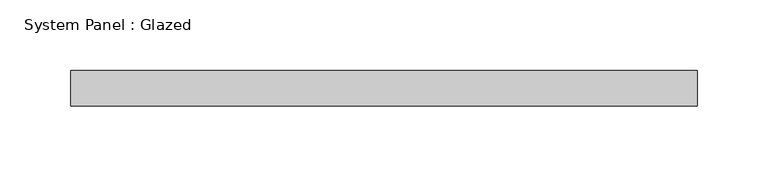
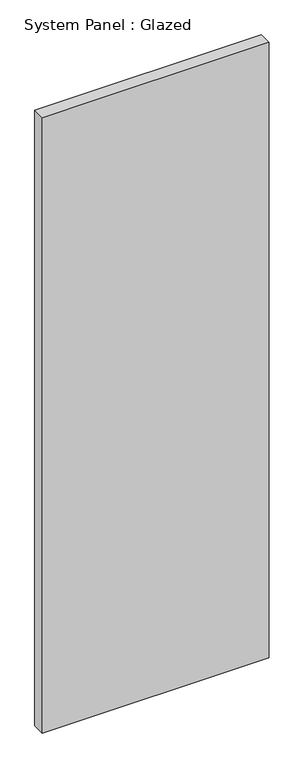
"""IFC4 building model written with IfcOpenShell, lengths in millimetres: plate geometry, System Panel : Glazed."""

from ifc_helpers import new_model, si_unit, origin, origin_with_axes, place, context, project, spatial, polyline, outline, extrude, source, transform, mapped, element, save


def system_panel_glazed_617ab36c(model_context):
    return source(origin(), model_context, "Body", "SweptSolid", [
        extrude(outline(polyline([(222.25, 19.05), (-222.25, 19.05), (-222.25, 44.45), (222.25, 44.45), (222.25, 19.05)])), origin_with_axes(), (0.0, 0.0, 1.0), 1274.633189),
    ])


if __name__ == "__main__":
    model = new_model("IFC4")
    model_context = context("Model", 3, world=origin())
    ifc_project = project(units=[si_unit("LENGTHUNIT", "METRE", prefix="MILLI")], contexts=[model_context])
    site = spatial("IfcSite", under=ifc_project)
    building = spatial("IfcBuilding", under=site)
    placement = place(None, origin())
    system_panel_glazed_shape = system_panel_glazed_617ab36c(model_context)
    element("IfcPlate", 1, ObjectType="System Panel : Glazed", at=placement, inside=building, context=model_context, shape_type="MappedRepresentation", body=[
        mapped(system_panel_glazed_shape, transform((0.0, 0.0, 0.0), x_axis=(1.0, 0.0, 0.0), y_axis=(0.0, 1.0, 0.0), z_axis=(0.0, 0.0, 1.0))),
    ])
    save(model, "model.ifc")

# Revit data of these elements
# Type "System Panel : Glazed"
#   Construction Type Id = "GSP4R"
#   Analytic Construction = "1/8 in Pilkington single glazing"
#   Visual Light Transmittance = 0.9
#   Solar Heat Gain Coefficient = 0.86
#   Heat Transfer Coefficient (U) = 1.18115 BTU/(h·ft²·°F)
#   Define Thermal Properties by = 1
# Element 1 (IfcPlate, "System Panel : Glazed")
#   Materials on its faces: "Glass"
# Materials
#   "Glass": class "Glass", colour RGB 0 128 192, transparency 0.75, Description = "Soda Lime Glass", Cost = 0
